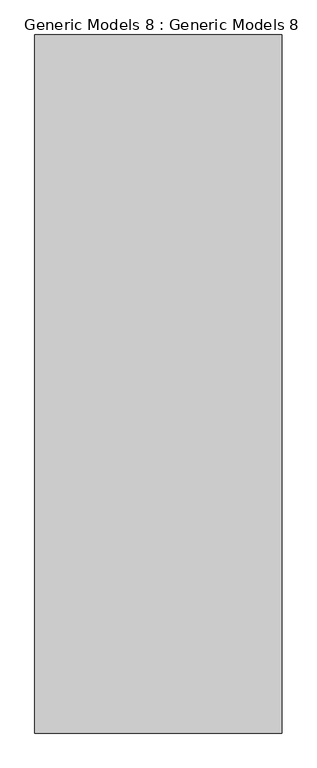
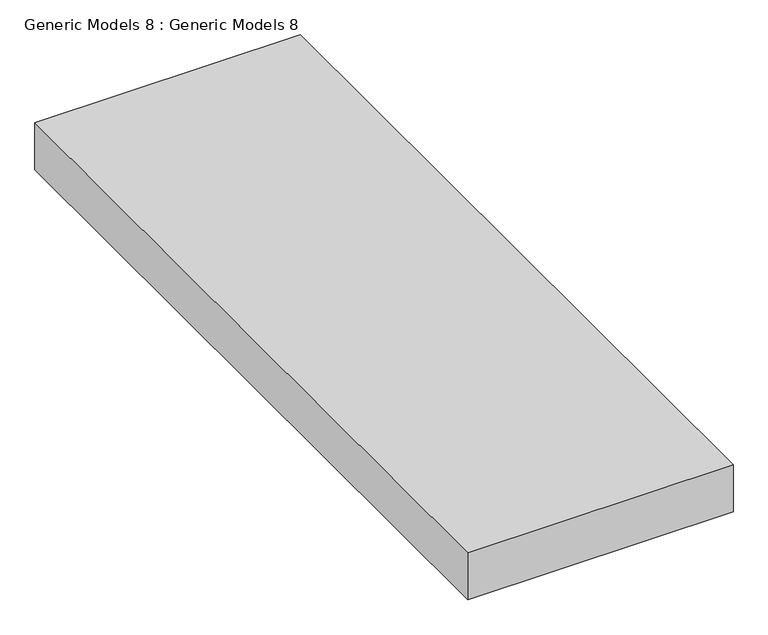
"""IFC4 building model written with IfcOpenShell, lengths in millimetres: proxy geometry, Generic Models 8 : Generic Models 8."""

from ifc_helpers import new_model, si_unit, frame, origin, place, context, project, spatial, polyline, outline, extrude, source, transform, mapped, element, save


def generic_models_8_generic_models_8_38ca69cf(model_context):
    return source(origin(), model_context, "Body", "SweptSolid", [
        extrude(outline(polyline([(-21035.2120831, 130.8673842), (-19816.0120831, 130.8673842), (-19816.0120831, -3312.1945627), (-21035.2120831, -3312.1945627), (-21035.2120831, 130.8673842)])), frame((0.0, 0.0, 2422.8588865), z_axis=(0.0, 0.0, 1.0), x_axis=(1.0, 0.0, 0.0)), (0.0, 0.0, 1.0), 228.6),
    ])


if __name__ == "__main__":
    model = new_model("IFC4")
    model_context = context("Model", 3, world=origin())
    ifc_project = project(units=[si_unit("LENGTHUNIT", "METRE", prefix="MILLI")], contexts=[model_context])
    site = spatial("IfcSite", under=ifc_project)
    building = spatial("IfcBuilding", under=site)
    placement = place(None, origin())
    generic_models_8_generic_models_8_shape = generic_models_8_generic_models_8_38ca69cf(model_context)
    element("IfcBuildingElementProxy", 1, Name="Generic Models 8 : Generic Models 8", ObjectType="Generic Models 8 : Generic Models 8", at=placement, inside=building, context=model_context, shape_type="MappedRepresentation", body=[
        mapped(generic_models_8_generic_models_8_shape, transform((0.0, 0.0, 0.0), x_axis=(1.0, 0.0, 0.0), y_axis=(0.0, 1.0, 0.0), z_axis=(0.0, 0.0, 1.0))),
    ])
    save(model, "model.ifc")
